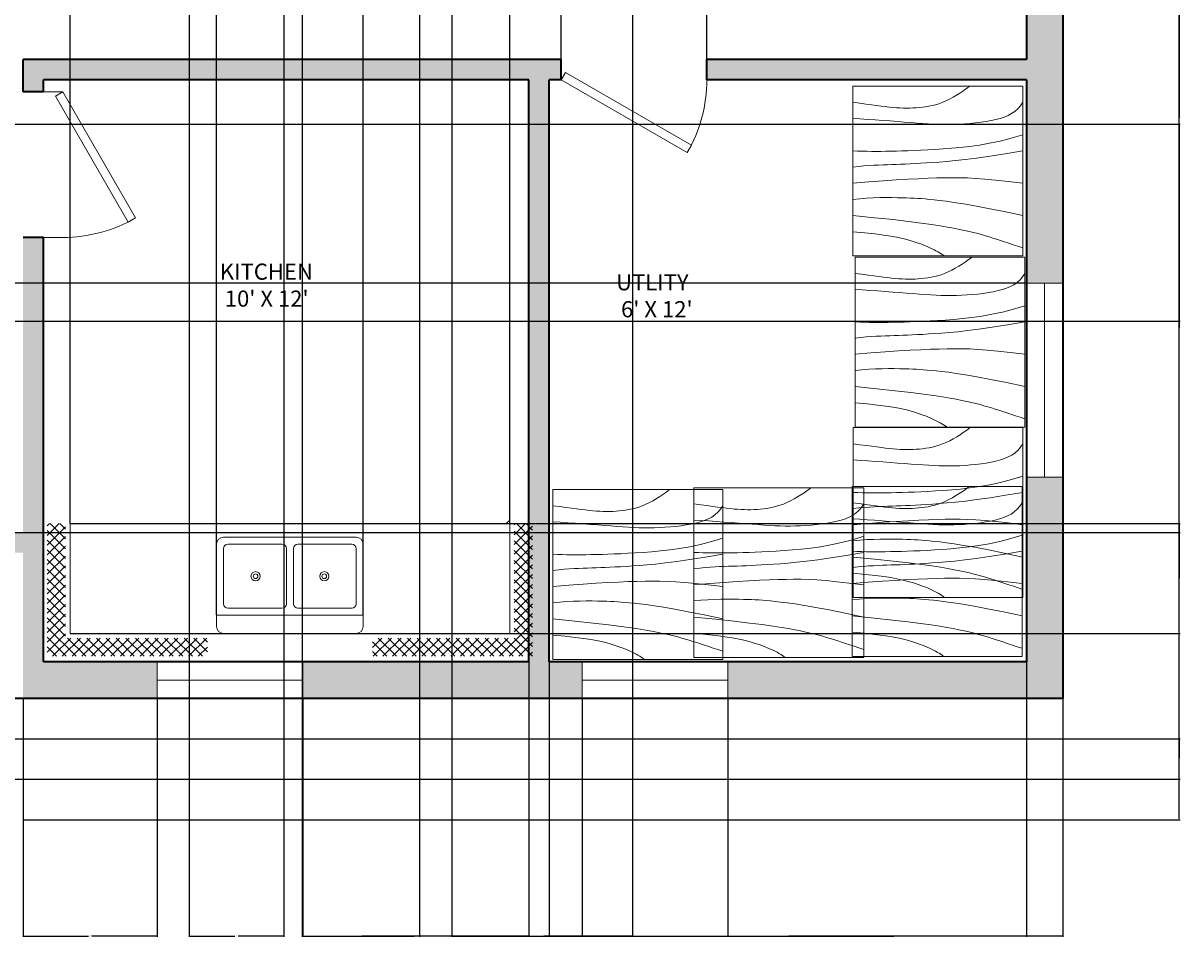
# Model space of a CAD drawing. Units: inches. Extents: x -28 to 649, y -11 to 509.
# Tile 5 of 7: x 346 to 633, y -11 to 215. Entities that reach past the tile are written whole.
import ezdxf

# ---------------------------------------------------------------- set-up
doc = ezdxf.new("R2010")
doc.units = ezdxf.units.IN
doc.header["$MEASUREMENT"] = 0
for name, color, linetype, lineweight in [('A-ANNO-DIMS', 2, 'Continuous', 18), ('A-AREA-IDEN', 18, 'Continuous', 18), ('A-FLOR-CASE', 4, 'Continuous', 20), ('A-FLOR-CASE-PATT', 181, 'Continuous', 13), ('A-FLOR-FIXT', 181, 'Continuous', 18), ('A-WALL', 7, 'Continuous', 35), ('A-WALL-PATT', 251, 'Continuous', 13), ('doors', 40, 'Continuous', 20), ('window', 30, 'Continuous', 18)]:
    doc.layers.add(name, color=color, linetype=linetype, lineweight=lineweight)
doc.styles.get("Standard").update_dxf_attribs({"font": 'arial.ttf'})
doc.dimstyles.get("Standard").update_dxf_attribs({"dimtxt": 0.18, "dimasz": 0.18, "dimexe": 0.18, "dimexo": 0.0625, "dimgap": 0.09, "dimtad": 0, "dimtih": 1, "dimtoh": 1, "dimdec": 4, "dimzin": 0, "dimdsep": 46, "dimtxsty": 'Standard', "dimcen": 0.09, "dimadec": 0, "dimazin": 0, "dimtfac": 1, "dimtdec": 4, "dimtofl": 0, "dimtmove": 0, "dimatfit": 3, "dimfxl": 1, "dimtolj": 1, "dimtzin": 0, "dimarcsym": 0})

# ---------------------------------------------------------------- blocks, each defined once
blk = doc.blocks.new('*U9')
for p, q in [((0, 0), (0, -100)), ((750, 0), (750, -100))]:
    blk.add_line(p, q)
blk.add_lwpolyline([(0, 0), (649.5, 375), (671.4, 337.1), (21.9, -37.9)], close=True)
blk.add_arc((0, 0), 750, 0, 30)
blk = doc.blocks.new('*U10')
for p, q in [((0, 0), (0, 100)), ((750, 0), (750, 100))]:
    blk.add_line(p, q)
blk.add_lwpolyline([(0, 0), (649.5, -375), (671.4, -337.1), (21.9, 37.9)], close=True)
blk.add_arc((0, 0), 750, 330, 0)
blk = doc.blocks.new('Table - Square Woodgrain 42 x 42 in.')
blk.add_line((0, -42), (42, -42))
for points in [[(0, -4), (1.704, -4.2172), (3.2358, -4.4188), (4.615, -4.604), (5.8615, -4.7721), (6.9951, -4.9224), (8.0357, -5.0541), (9.0031, -5.1667), (9.9171, -5.2594), (10.7951, -5.3316), (11.6445, -5.3836), (12.4702, -5.4157), (13.277, -5.4283), (14.0698, -5.4217), (14.8535, -5.3964), (15.6331, -5.3526), (16.4133, -5.2908), (17.1986, -5.2103), (17.9913, -5.1062), (18.793, -4.9727), (19.6056, -4.8038), (20.4307, -4.5937), (21.2701, -4.3365), (22.1256, -4.0262), (22.9989, -3.6571), (23.888, -3.2272), (24.7756, -2.7516), (25.6408, -2.2491), (26.4624, -1.7387), (27.2195, -1.2395), (27.891, -0.7703), (28.456, -0.3501), (28.8934, 0.002)], [(0, -42), (0, 0), (42, 0), (42, -42)], [(0, -8), (1.8203, -8.1001), (3.6741, -8.2149), (5.5411, -8.3408), (7.4011, -8.4741), (9.2339, -8.6112), (11.0193, -8.7484), (12.7371, -8.8821), (14.3671, -9.0086), (15.8954, -9.1246), (17.3337, -9.2278), (18.6997, -9.3159), (20.0116, -9.387), (21.2871, -9.4389), (22.5442, -9.4696), (23.8008, -9.477), (25.0749, -9.459), (26.3791, -9.4137), (27.7049, -9.3403), (29.0383, -9.2382), (30.3655, -9.1068), (31.6728, -8.9455), (32.9461, -8.7535), (34.1717, -8.5304), (35.3358, -8.2756), (36.4268, -7.9863), (37.443, -7.6521), (38.3849, -7.2603), (39.253, -6.7986), (40.048, -6.2542), (40.7705, -5.6147), (41.421, -4.8674), (42, -4)], [(42, -12), (39.1784, -12.8621), (36.4519, -13.5654), (33.8246, -14.1294), (31.3004, -14.5731), (28.8832, -14.9161), (26.577, -15.1775), (24.3858, -15.3768), (22.3136, -15.5332), (20.3622, -15.6632), (18.5254, -15.7718), (16.7947, -15.8612), (15.1618, -15.9338), (13.6183, -15.9916), (12.1558, -16.0369), (10.7659, -16.0718), (9.4403, -16.0987), (8.1703, -16.1191), (6.9461, -16.1325), (5.7577, -16.1377), (4.595, -16.1335), (3.4479, -16.1188), (2.3064, -16.0924), (1.1604, -16.0532), (0, -16)], [(42, -16), (37.6529, -16.7365), (33.8802, -17.329), (30.6179, -17.7961), (27.8015, -18.1561), (25.3668, -18.4275), (23.2497, -18.6288), (21.3859, -18.7785), (19.7111, -18.8949), (18.1693, -18.9939), (16.7375, -19.0795), (15.401, -19.1534), (14.1449, -19.217), (12.9544, -19.2717), (11.8148, -19.3191), (10.7113, -19.3606), (9.6291, -19.3976), (8.5534, -19.4323), (7.47, -19.4689), (6.3643, -19.5122), (5.222, -19.5672), (4.0288, -19.6386), (2.7703, -19.7313), (1.4321, -19.8501), (0, -20)], [(0, -24), (3.9243, -23.6805), (7.4766, -23.4138), (10.6891, -23.1954), (13.5943, -23.0205), (16.2247, -22.8847), (18.6125, -22.7832), (20.7903, -22.7116), (22.7903, -22.6651), (24.6563, -22.642), (26.4764, -22.6507), (28.35, -22.7024), (30.3766, -22.8084), (32.6555, -22.98), (35.2861, -23.2283), (38.3678, -23.5645), (42, -24)], [(42, -32), (37.392, -31.017), (33.4585, -30.2231), (30.1291, -29.5949), (27.3334, -29.109), (25.0009, -28.742), (23.0612, -28.4707), (21.4439, -28.2716), (20.0786, -28.1215), (18.8998, -28.0002), (17.8609, -27.9014), (16.9206, -27.8219), (16.0371, -27.7588), (15.1691, -27.709), (14.2748, -27.6693), (13.3128, -27.6368), (12.2415, -27.6083), (11.0295, -27.5824), (9.6867, -27.5643), (8.233, -27.5608), (6.6884, -27.5787), (5.0728, -27.6248), (3.4062, -27.7058), (1.7086, -27.8286), (0, -28)], [(0, -32), (5.4026, -32.5358), (9.9494, -33.019), (13.7424, -33.4553), (16.8834, -33.8505), (19.4743, -34.2106), (21.6171, -34.5413), (23.4136, -34.8486), (24.9657, -35.1382), (26.3614, -35.4156), (27.6332, -35.6841), (28.7995, -35.9467), (29.8788, -36.2064), (30.8897, -36.4661), (31.8507, -36.7288), (32.7802, -36.9973), (33.6968, -37.2747), (34.6175, -37.5635), (35.5531, -37.8651), (36.5128, -38.1805), (37.506, -38.5108), (38.5421, -38.8568), (39.6302, -39.2197), (40.7797, -39.6004), (42, -40)], [(0, -36), (3.0098, -36.2857), (5.5354, -36.5643), (7.6368, -36.8359), (9.374, -37.1009), (10.807, -37.3597), (11.9957, -37.6126), (13.0002, -37.8599), (13.8804, -38.102), (14.6874, -38.3393), (15.4365, -38.5729), (16.1338, -38.8041), (16.7858, -39.0341), (17.3987, -39.264), (17.9787, -39.4952), (18.5322, -39.7288), (19.0655, -39.9662), (19.5832, -40.2081), (20.0842, -40.4544), (20.5657, -40.7046), (21.0249, -40.9581), (21.459, -41.2144), (21.8653, -41.4731), (22.2409, -41.7335), (22.5831, -41.9951)]]:
    blk.add_lwpolyline(points)
blk = doc.blocks.new('WIN-48x9')
for p, q in [((9, 48), (0, 48)), ((0, 48), (0, 0)), ((4.5, 0), (4.5, 48)), ((9, 0), (9, 48)), ((0, 0), (9, 0)), ((0, 0), (4.5, 0))]:
    blk.add_line(p, q)
blk = doc.blocks.new('WIN-36x9')
for p, q in [((0, 9), (0, 0)), ((36, 9), (0, 9)), ((0, 9), (0, 4.5)), ((36, 0), (36, 9)), ((0, 4.5), (36, 4.5)), ((0, 0), (36, 0))]:
    blk.add_line(p, q)
blk = doc.blocks.new('*D31')
at = {"layer": 'A-ANNO-DIMS', "color": 0, "lineweight": -2, "transparency": 16777216}
for p, q in [((603.51, 479.94), (632.43, 479.94)), ((632.25, 479.76), (632.25, 249.12)), ((632.25, 18.12), (632.25, 248.76)), ((346.51, 17.94), (632.43, 17.94))]:
    blk.add_line(p, q, dxfattribs=at)
at = {"layer": 'A-ANNO-DIMS', "color": 0, "transparency": 16777216}
for points in [[(632.22, 479.76), (632.28, 479.76), (632.25, 479.94)], [(632.22, 18.12), (632.28, 18.12), (632.25, 17.94)]]:
    blk.add_solid(points, dxfattribs=at)
at = {"layer": 'Defpoints', "color": 0, "transparency": 16777216}
for p in [(603.45, 479.94), (632.25, 479.94), (346.45, 17.94)]:
    blk.add_point(p, dxfattribs=at)
at = {"layer": 'A-ANNO-DIMS', "color": 0, "transparency": 16777216, "insert": (632.25, 248.94), "char_height": 0.18, "attachment_point": 5}
blk.add_mtext('\\A1;462', dxfattribs=at)
blk = doc.blocks.new('*D33')
at = {"layer": 'A-ANNO-DIMS', "color": 0, "lineweight": -2, "transparency": 16777216}
for p, q in [((280.51, 37.94), (632.43, 37.94)), ((632.25, 37.76), (632.25, 33.12)), ((632.25, 28.12), (632.25, 32.76)), ((280.51, 27.94), (632.43, 27.94))]:
    blk.add_line(p, q, dxfattribs=at)
at = {"layer": 'A-ANNO-DIMS', "color": 0, "transparency": 16777216}
for points in [[(632.22, 37.76), (632.28, 37.76), (632.25, 37.94)], [(632.22, 28.12), (632.28, 28.12), (632.25, 27.94)]]:
    blk.add_solid(points, dxfattribs=at)
at = {"layer": 'Defpoints', "color": 0, "transparency": 16777216}
for p in [(280.45, 37.94), (632.25, 37.94), (280.45, 27.94)]:
    blk.add_point(p, dxfattribs=at)
at = {"layer": 'A-ANNO-DIMS', "color": 0, "transparency": 16777216, "insert": (632.25, 32.94), "char_height": 0.18, "attachment_point": 5}
blk.add_mtext('\\A1;10', dxfattribs=at)
blk = doc.blocks.new('*D40')
at = {"layer": 'A-ANNO-DIMS', "color": 0, "lineweight": -2, "transparency": 16777216}
for p, q in [((346.45, 47.88), (346.45, -11.04)), ((379.58, 47.88), (379.58, -11.04)), ((346.63, -10.86), (362.62, -10.86)), ((379.4, -10.86), (363.41, -10.86))]:
    blk.add_line(p, q, dxfattribs=at)
at = {"layer": 'A-ANNO-DIMS', "color": 0, "transparency": 16777216}
for points in [[(346.63, -10.83), (346.63, -10.89), (346.45, -10.86)], [(379.4, -10.83), (379.4, -10.89), (379.58, -10.86)]]:
    blk.add_solid(points, dxfattribs=at)
at = {"layer": 'Defpoints', "color": 0, "transparency": 16777216}
for p in [(346.45, 47.94), (379.58, 47.94), (379.58, -10.86)]:
    blk.add_point(p, dxfattribs=at)
at = {"layer": 'A-ANNO-DIMS', "color": 0, "transparency": 16777216, "insert": (363.01, -10.86), "char_height": 0.18, "attachment_point": 5}
blk.add_mtext('\\A1;33.13', dxfattribs=at)
blk = doc.blocks.new('*D41')
at = {"layer": 'A-ANNO-DIMS', "color": 0, "lineweight": -2, "transparency": 16777216}
for p, q in [((471.45, 56.88), (471.45, -11.04)), ((415.58, 47.88), (415.58, -11.04)), ((415.76, -10.86), (443.12, -10.86)), ((471.27, -10.86), (443.91, -10.86))]:
    blk.add_line(p, q, dxfattribs=at)
at = {"layer": 'A-ANNO-DIMS', "color": 0, "transparency": 16777216}
for points in [[(415.76, -10.83), (415.76, -10.89), (415.58, -10.86)], [(471.27, -10.83), (471.27, -10.89), (471.45, -10.86)]]:
    blk.add_solid(points, dxfattribs=at)
at = {"layer": 'Defpoints', "color": 0, "transparency": 16777216}
for p in [(471.45, 56.94), (415.58, 47.94), (471.45, -10.86)]:
    blk.add_point(p, dxfattribs=at)
at = {"layer": 'A-ANNO-DIMS', "color": 0, "transparency": 16777216, "insert": (443.51, -10.86), "char_height": 0.18, "attachment_point": 5}
blk.add_mtext('\\A1;55.87', dxfattribs=at)
blk = doc.blocks.new('*D42')
at = {"layer": 'A-ANNO-DIMS', "color": 0, "lineweight": -2, "transparency": 16777216}
for p, q in [((471.45, 56.88), (471.45, -11.04)), ((484.62, 47.88), (484.62, -11.04)), ((471.63, -10.86), (477.58, -10.86)), ((484.44, -10.86), (478.49, -10.86))]:
    blk.add_line(p, q, dxfattribs=at)
at = {"layer": 'A-ANNO-DIMS', "color": 0, "transparency": 16777216}
for points in [[(471.63, -10.83), (471.63, -10.89), (471.45, -10.86)], [(484.44, -10.83), (484.44, -10.89), (484.62, -10.86)]]:
    blk.add_solid(points, dxfattribs=at)
at = {"layer": 'Defpoints', "color": 0, "transparency": 16777216}
for p in [(471.45, 56.94), (484.62, 47.94), (484.62, -10.86)]:
    blk.add_point(p, dxfattribs=at)
at = {"layer": 'A-ANNO-DIMS', "color": 0, "transparency": 16777216, "insert": (478.03, -10.86), "char_height": 0.18, "attachment_point": 5}
blk.add_mtext('\\A1;13.168', dxfattribs=at)
blk = doc.blocks.new('*D43')
at = {"layer": 'A-ANNO-DIMS', "color": 0, "lineweight": -2, "transparency": 16777216}
for p, q in [((520.62, 47.88), (520.62, -11.04)), ((603.45, 47.88), (603.45, -11.04)), ((520.8, -10.86), (561.64, -10.86)), ((603.27, -10.86), (562.43, -10.86))]:
    blk.add_line(p, q, dxfattribs=at)
at = {"layer": 'A-ANNO-DIMS', "color": 0, "transparency": 16777216}
for points in [[(520.8, -10.83), (520.8, -10.89), (520.62, -10.86)], [(603.27, -10.83), (603.27, -10.89), (603.45, -10.86)]]:
    blk.add_solid(points, dxfattribs=at)
at = {"layer": 'Defpoints', "color": 0, "transparency": 16777216}
for p in [(520.62, 47.94), (603.45, 47.94), (603.45, -10.86)]:
    blk.add_point(p, dxfattribs=at)
at = {"layer": 'A-ANNO-DIMS', "color": 0, "transparency": 16777216, "insert": (562.03, -10.86), "char_height": 0.18, "attachment_point": 5}
blk.add_mtext('\\A1;82.83', dxfattribs=at)
blk = doc.blocks.new('*D47')
at = {"layer": 'A-ANNO-DIMS', "color": 0, "lineweight": -2, "transparency": 16777216}
for p, q in [((387.45, 470.88), (387.45, -11.04)), ((410.91, 470.88), (410.91, -11.04)), ((387.63, -10.86), (398.79, -10.86)), ((410.73, -10.86), (399.58, -10.86))]:
    blk.add_line(p, q, dxfattribs=at)
at = {"layer": 'A-ANNO-DIMS', "color": 0, "transparency": 16777216}
for points in [[(387.63, -10.83), (387.63, -10.89), (387.45, -10.86)], [(410.73, -10.83), (410.73, -10.89), (410.91, -10.86)]]:
    blk.add_solid(points, dxfattribs=at)
at = {"layer": 'Defpoints', "color": 0, "transparency": 16777216}
for p in [(387.45, 470.94), (410.91, 470.94), (410.91, -10.86)]:
    blk.add_point(p, dxfattribs=at)
at = {"layer": 'A-ANNO-DIMS', "color": 0, "transparency": 16777216, "insert": (399.18, -10.86), "char_height": 0.18, "attachment_point": 5}
blk.add_mtext('\\A1;23.46', dxfattribs=at)
blk = doc.blocks.new('*D48')
at = {"layer": 'A-ANNO-DIMS', "color": 0, "lineweight": -2, "transparency": 16777216}
for p, q in [((452.45, 470.88), (452.45, -11.04)), ((497.1, 470.88), (497.1, -11.04)), ((452.63, -10.86), (474.38, -10.86)), ((496.92, -10.86), (475.17, -10.86))]:
    blk.add_line(p, q, dxfattribs=at)
at = {"layer": 'A-ANNO-DIMS', "color": 0, "transparency": 16777216}
for points in [[(452.63, -10.83), (452.63, -10.89), (452.45, -10.86)], [(496.92, -10.83), (496.92, -10.89), (497.1, -10.86)]]:
    blk.add_solid(points, dxfattribs=at)
at = {"layer": 'Defpoints', "color": 0, "transparency": 16777216}
for p in [(452.45, 470.94), (497.1, 470.94), (497.1, -10.86)]:
    blk.add_point(p, dxfattribs=at)
at = {"layer": 'A-ANNO-DIMS', "color": 0, "transparency": 16777216, "insert": (474.77, -10.86), "char_height": 0.18, "attachment_point": 5}
blk.add_mtext('\\A1;44.65', dxfattribs=at)
blk = doc.blocks.new('*D52')
at = {"layer": 'A-ANNO-DIMS', "color": 0, "lineweight": -2, "transparency": 16777216}
for p, q in [((594.39, 262.25), (-1.53, 262.25)), ((-1.35, 262.07), (-1.35, 206.61)), ((-1.35, 150.79), (-1.35, 206.25)), ((594.39, 150.61), (-1.53, 150.61))]:
    blk.add_line(p, q, dxfattribs=at)
at = {"layer": 'A-ANNO-DIMS', "color": 0, "transparency": 16777216}
for points in [[(-1.38, 262.07), (-1.32, 262.07), (-1.35, 262.25)], [(-1.38, 150.79), (-1.32, 150.79), (-1.35, 150.61)]]:
    blk.add_solid(points, dxfattribs=at)
at = {"layer": 'Defpoints', "color": 0, "transparency": 16777216}
for p in [(-1.35, 262.25), (594.45, 262.25), (594.45, 150.61)]:
    blk.add_point(p, dxfattribs=at)
at = {"layer": 'A-ANNO-DIMS', "color": 0, "transparency": 16777216, "insert": (-1.35, 206.43), "char_height": 0.18, "attachment_point": 5}
blk.add_mtext('\\A1;111.64', dxfattribs=at)
blk = doc.blocks.new('*D53')
at = {"layer": 'A-ANNO-DIMS', "color": 0, "lineweight": -2, "transparency": 16777216}
for p, q in [((36.51, 241.9), (632.43, 241.9)), ((632.25, 241.72), (632.25, 191.76)), ((632.25, 141.44), (632.25, 191.39)), ((36.51, 141.26), (632.43, 141.26))]:
    blk.add_line(p, q, dxfattribs=at)
at = {"layer": 'A-ANNO-DIMS', "color": 0, "transparency": 16777216}
for points in [[(632.22, 241.72), (632.28, 241.72), (632.25, 241.9)], [(632.22, 141.44), (632.28, 141.44), (632.25, 141.26)]]:
    blk.add_solid(points, dxfattribs=at)
at = {"layer": 'Defpoints', "color": 0, "transparency": 16777216}
for p in [(36.45, 241.9), (632.25, 241.9), (36.45, 141.26)]:
    blk.add_point(p, dxfattribs=at)
at = {"layer": 'A-ANNO-DIMS', "color": 0, "transparency": 16777216, "insert": (632.25, 191.58), "char_height": 0.18, "attachment_point": 5}
blk.add_mtext('\\A1;100.64', dxfattribs=at)
blk = doc.blocks.new('*D60')
at = {"layer": 'A-ANNO-DIMS', "color": 0, "lineweight": -2, "transparency": 16777216}
for p, q in [((479.45, 206), (479.45, 508.92)), ((479.63, 508.74), (497.23, 508.74)), ((515.27, 508.74), (497.67, 508.74)), ((515.45, 206), (515.45, 508.92))]:
    blk.add_line(p, q, dxfattribs=at)
at = {"layer": 'A-ANNO-DIMS', "color": 0, "transparency": 16777216}
for points in [[(479.63, 508.77), (479.63, 508.71), (479.45, 508.74)], [(515.27, 508.77), (515.27, 508.71), (515.45, 508.74)]]:
    blk.add_solid(points, dxfattribs=at)
at = {"layer": 'Defpoints', "color": 0, "transparency": 16777216}
for p in [(515.45, 508.74), (479.45, 205.94), (515.45, 205.94)]:
    blk.add_point(p, dxfattribs=at)
at = {"layer": 'A-ANNO-DIMS', "color": 0, "transparency": 16777216, "insert": (497.45, 508.74), "char_height": 0.18, "attachment_point": 5}
blk.add_mtext('\\A1;36', dxfattribs=at)
blk = doc.blocks.new('*D61')
at = {"layer": 'A-ANNO-DIMS', "color": 0, "lineweight": -2, "transparency": 16777216}
for p, q in [((274.51, 189.94), (632.43, 189.94)), ((632.25, 189.76), (632.25, 139.62)), ((632.25, 89.12), (632.25, 139.26)), ((274.51, 88.94), (632.43, 88.94))]:
    blk.add_line(p, q, dxfattribs=at)
at = {"layer": 'A-ANNO-DIMS', "color": 0, "transparency": 16777216}
for points in [[(632.22, 189.76), (632.28, 189.76), (632.25, 189.94)], [(632.22, 89.12), (632.28, 89.12), (632.25, 88.94)]]:
    blk.add_solid(points, dxfattribs=at)
at = {"layer": 'Defpoints', "color": 0, "transparency": 16777216}
for p in [(274.45, 189.94), (632.25, 189.94), (274.45, 88.94)]:
    blk.add_point(p, dxfattribs=at)
at = {"layer": 'A-ANNO-DIMS', "color": 0, "transparency": 16777216, "insert": (632.25, 139.44), "char_height": 0.18, "attachment_point": 5}
blk.add_mtext('\\A1;101', dxfattribs=at)
blk = doc.blocks.new('*D63')
at = {"layer": 'A-ANNO-DIMS', "color": 0, "lineweight": -2, "transparency": 16777216}
for p, q in [((415.45, 381.88), (415.45, -11.04)), ((444.45, 381.88), (444.45, -11.04)), ((415.63, -10.86), (429.73, -10.86)), ((444.27, -10.86), (430.17, -10.86))]:
    blk.add_line(p, q, dxfattribs=at)
at = {"layer": 'A-ANNO-DIMS', "color": 0, "transparency": 16777216}
for points in [[(415.63, -10.83), (415.63, -10.89), (415.45, -10.86)], [(444.27, -10.83), (444.27, -10.89), (444.45, -10.86)]]:
    blk.add_solid(points, dxfattribs=at)
at = {"layer": 'Defpoints', "color": 0, "transparency": 16777216}
for p in [(415.45, 381.94), (444.45, 381.94), (444.45, -10.86)]:
    blk.add_point(p, dxfattribs=at)
at = {"layer": 'A-ANNO-DIMS', "color": 0, "transparency": 16777216, "insert": (429.95, -10.86), "char_height": 0.18, "attachment_point": 5}
blk.add_mtext('\\A1;29', dxfattribs=at)
blk = doc.blocks.new('*D68')
at = {"layer": 'A-ANNO-DIMS', "color": 0, "lineweight": -2, "transparency": 16777216}
for p, q in [((358.05, 91.23), (358.05, 508.92)), ((358.23, 508.74), (411.94, 508.74)), ((466.55, 508.74), (412.85, 508.74)), ((466.73, 91.23), (466.73, 508.92))]:
    blk.add_line(p, q, dxfattribs=at)
at = {"layer": 'A-ANNO-DIMS', "color": 0, "transparency": 16777216}
for points in [[(358.23, 508.77), (358.23, 508.71), (358.05, 508.74)], [(466.55, 508.77), (466.55, 508.71), (466.73, 508.74)]]:
    blk.add_solid(points, dxfattribs=at)
at = {"layer": 'Defpoints', "color": 0, "transparency": 16777216}
for p in [(466.73, 508.74), (358.05, 91.17), (466.73, 91.17)]:
    blk.add_point(p, dxfattribs=at)
at = {"layer": 'A-ANNO-DIMS', "color": 0, "transparency": 16777216, "insert": (412.39, 508.74), "char_height": 0.18, "attachment_point": 5}
blk.add_mtext('\\A1;108.68', dxfattribs=at)
blk = doc.blocks.new('*D69')
at = {"layer": 'A-ANNO-DIMS', "color": 0, "lineweight": -2, "transparency": 16777216}
for p, q in [((358.11, 91.17), (632.43, 91.17)), ((632.25, 90.99), (632.25, 77.76)), ((632.25, 64.18), (632.25, 77.4)), ((358.11, 64), (632.43, 64))]:
    blk.add_line(p, q, dxfattribs=at)
at = {"layer": 'A-ANNO-DIMS', "color": 0, "transparency": 16777216}
for points in [[(632.22, 90.99), (632.28, 90.99), (632.25, 91.17)], [(632.22, 64.18), (632.28, 64.18), (632.25, 64)]]:
    blk.add_solid(points, dxfattribs=at)
at = {"layer": 'Defpoints', "color": 0, "transparency": 16777216}
for p in [(358.05, 91.17), (632.25, 91.17), (358.05, 64)]:
    blk.add_point(p, dxfattribs=at)
at = {"layer": 'A-ANNO-DIMS', "color": 0, "transparency": 16777216, "insert": (632.25, 77.58), "char_height": 0.18, "attachment_point": 5}
blk.add_mtext('\\A1;27.17', dxfattribs=at)
blk = doc.blocks.new('*D70')
at = {"layer": 'A-ANNO-DIMS', "color": 0, "lineweight": -2, "transparency": 16777216}
for p, q in [((394.28, 68.59), (394.28, 508.92)), ((394.46, 508.74), (412, 508.74)), ((430.33, 508.74), (412.79, 508.74)), ((430.51, 68.59), (430.51, 508.92))]:
    blk.add_line(p, q, dxfattribs=at)
at = {"layer": 'A-ANNO-DIMS', "color": 0, "transparency": 16777216}
for points in [[(394.46, 508.77), (394.46, 508.71), (394.28, 508.74)], [(430.33, 508.77), (430.33, 508.71), (430.51, 508.74)]]:
    blk.add_solid(points, dxfattribs=at)
at = {"layer": 'Defpoints', "color": 0, "transparency": 16777216}
for p in [(430.51, 508.74), (394.28, 68.53), (430.51, 68.53)]:
    blk.add_point(p, dxfattribs=at)
at = {"layer": 'A-ANNO-DIMS', "color": 0, "transparency": 16777216, "insert": (412.39, 508.74), "char_height": 0.18, "attachment_point": 5}
blk.add_mtext('\\A1;36.23', dxfattribs=at)
blk = doc.blocks.new('*D71')
at = {"layer": 'A-ANNO-DIMS', "color": 0, "lineweight": -2, "transparency": 16777216}
for p, q in [((476.45, 56.88), (476.45, -11.04)), ((594.45, 56.88), (594.45, -11.04)), ((476.63, -10.86), (535.17, -10.86)), ((594.27, -10.86), (535.73, -10.86))]:
    blk.add_line(p, q, dxfattribs=at)
at = {"layer": 'A-ANNO-DIMS', "color": 0, "transparency": 16777216}
for points in [[(476.63, -10.83), (476.63, -10.89), (476.45, -10.86)], [(594.27, -10.83), (594.27, -10.89), (594.45, -10.86)]]:
    blk.add_solid(points, dxfattribs=at)
at = {"layer": 'Defpoints', "color": 0, "transparency": 16777216}
for p in [(476.45, 56.94), (594.45, 56.94), (594.45, -10.86)]:
    blk.add_point(p, dxfattribs=at)
at = {"layer": 'A-ANNO-DIMS', "color": 0, "transparency": 16777216, "insert": (535.45, -10.86), "char_height": 0.18, "attachment_point": 5}
blk.add_mtext('\\A1;118', dxfattribs=at)

msp = doc.modelspace()

# ---------------------------------------------------------------- hatches: boundary and pattern name
at = {"layer": 'A-FLOR-CASE-PATT'}
h = msp.add_hatch(dxfattribs=at)
h.set_pattern_fill('ANSI37', color=256, scale=13.5849, style=0)
h.paths.add_polyline_path([(352.3918, 58.3392), (392.0145, 58.3392), (392.0145, 62.8675), (356.9201, 62.8675), (356.9201, 91.1694), (352.3918, 91.1694)])
h = msp.add_hatch(dxfattribs=at)
h.set_pattern_fill('ANSI37', color=256, scale=13.5849, style=0)
h.paths.add_polyline_path([(432.7692, 58.3392), (472.3918, 58.3392), (472.3918, 91.1694), (467.8635, 91.1694), (467.8635, 62.8675), (432.7692, 62.8675)])
at = {"layer": 'A-WALL-PATT'}
h = msp.add_hatch(color=256, dxfattribs=at)
h.dxf.hatch_style = 1
h.paths.add_polyline_path([(36.4499, 184.9382), (165.4499, 184.9382), (165.4499, 189.9382), (36.4499, 189.9382), (36.4499, 241.898), (27.4499, 241.898), (27.4499, 141.2558), (36.4499, 141.2558)])
h.paths.add_polyline_path([(36.4499, 385.8835), (27.4499, 385.8835), (27.4499, 289.898), (36.4499, 289.898)])
h.paths.add_polyline_path([(185.4499, 341.9382), (180.4499, 341.9382), (180.4499, 338.9382), (36.4499, 338.9382), (36.4499, 333.9382), (185.4499, 333.9382)])
h.paths.add_polyline_path([(36.4499, 470.9382), (79.2168, 470.9382), (79.2168, 479.9382), (27.4499, 479.9382), (27.4499, 433.8835), (36.4499, 433.8835)])
h.paths.add_polyline_path([(185.4499, 470.9382), (203.9104, 470.9382), (203.9104, 479.9382), (127.2168, 479.9382), (127.2168, 470.9382), (180.4499, 470.9382), (180.4499, 381.9382), (188.4499, 381.9382), (188.4499, 386.9382), (185.4499, 386.9382)])
h.paths.add_polyline_path([(292.4601, 479.9382), (227.9104, 479.9382), (227.9104, 470.9382), (245.4499, 470.9382), (245.4499, 386.9382), (217.4499, 386.9382), (217.4499, 381.9382), (245.4499, 381.9382), (245.4499, 338.9382), (245.4499, 333.9382), (251.5222, 333.9382), (251.5222, 338.9382), (250.4499, 338.9382), (250.4499, 470.9382), (292.4601, 470.9382)])
h.paths.add_polyline_path([(410.9121, 479.9382), (340.4601, 479.9382), (340.4601, 470.9382), (382.4499, 470.9382), (382.4499, 338.9382), (287.5222, 338.9382), (287.5222, 333.9382), (387.4499, 333.9382), (387.4499, 381.9382), (415.4499, 381.9382), (415.4499, 386.9382), (387.4499, 386.9382), (387.4499, 470.9382), (410.9121, 470.9382)])
h.paths.add_polyline_path([(497.0961, 479.9382), (434.9121, 479.9382), (434.9121, 470.9382), (447.4499, 470.9382), (447.4499, 386.9382), (444.4499, 386.9382), (444.4499, 381.9382), (452.4499, 381.9382), (452.4499, 470.9382), (497.0961, 470.9382)])
h.paths.add_polyline_path([(603.4499, 479.9382), (545.0961, 479.9382), (545.0961, 470.9382), (594.4499, 470.9382), (594.4499, 418.4819), (603.4499, 418.4819)])
h.paths.add_polyline_path([(603.4499, 370.4819), (594.4499, 370.4819), (594.4499, 338.9382), (452.4499, 338.9382), (452.4499, 341.9382), (447.4499, 341.9382), (447.4499, 338.9382), (447.4499, 333.9382), (594.4499, 333.9382), (594.4499, 310.2528), (603.4499, 310.2528)])
h.paths.add_polyline_path([(603.4499, 262.2528), (594.4499, 262.2528), (594.4499, 205.9382), (515.4499, 205.9382), (515.4499, 200.9382), (594.4499, 200.9382), (594.4499, 150.6102), (603.4499, 150.6102)])
h = msp.add_hatch(color=256, dxfattribs=at)
h.dxf.hatch_style = 1
h.paths.add_polyline_path([(603.4499, 102.6102), (594.4499, 102.6102), (594.4499, 56.9382), (520.6175, 56.9382), (520.6175, 47.9382), (603.4499, 47.9382)])
h.paths.add_polyline_path([(484.6175, 56.9382), (476.4499, 56.9382), (476.4499, 200.9382), (479.4499, 200.9382), (479.4499, 205.9382), (346.4499, 205.9382), (346.4499, 197.9382), (351.4499, 197.9382), (351.4499, 200.9382), (471.4499, 200.9382), (471.4499, 56.9382), (415.5771, 56.9382), (415.5771, 47.9382), (484.6175, 47.9382)])
h.paths.add_polyline_path([(379.5771, 56.9382), (351.4499, 56.9382), (351.4499, 161.9382), (346.4499, 161.9382), (346.4499, 88.9382), (334.4499, 88.9382), (334.4499, 83.9382), (346.4499, 83.9382), (346.4499, 47.9382), (379.5771, 47.9382)])

# ---------------------------------------------------------------- linework, layer by layer
at = {"layer": 'A-FLOR-CASE'}
msp.add_lwpolyline([(466.7314, 91.1694), (466.7314, 63.9996), (358.0522, 63.9996), (358.0522, 91.1694)], close=True, dxfattribs=at)
at = {"layer": 'A-FLOR-CASE-PATT'}
msp.add_line((465.8821, 91.1694), (466.7314, 92.0187), dxfattribs=at)
at = {"layer": 'A-FLOR-FIXT'}
msp.add_line((430.505, 68.5279), (394.2786, 68.5279), dxfattribs=at)
for points in [[(430.505, 65.6977, -0.41421356), (428.8069, 63.9996), (395.9767, 63.9996, -0.41421356), (394.2786, 65.6977), (394.2786, 86.075, -0.41421356), (395.9767, 87.7732), (428.8069, 87.7732, -0.41421356), (430.505, 86.075)], [(397.1088, 70.226, -0.41421356), (395.9767, 71.3581), (395.9767, 84.943, -0.41421356), (397.1088, 86.075), (410.4107, 86.075, -0.41421356), (411.5428, 84.943), (411.5428, 71.3581, -0.41421356), (410.4107, 70.226)], [(413.2409, 84.943, -0.41421356), (414.3729, 86.075), (427.6748, 86.075, -0.41421356), (428.8069, 84.943), (428.8069, 71.3581, -0.41421356), (427.6748, 70.226), (414.3729, 70.226, -0.41421356), (413.2409, 71.3581)]]:
    msp.add_lwpolyline(points, format="xyb", close=True, dxfattribs=at)
for centre, radius in [((403.9012, 78.1505), 1.1321), ((403.9012, 78.1505), 0.566), ((420.8824, 78.1505), 1.1321), ((420.8824, 78.1505), 0.566)]:
    msp.add_circle(centre, radius, dxfattribs=at)
at = {"layer": 'A-WALL'}
for p, q in [((594.4499, 333.9382), (594.4499, 205.9382)), ((479.4499, 205.9382), (346.4499, 205.9382)), ((346.4499, 197.9382), (346.4499, 205.9382)), ((479.4499, 200.9382), (479.4499, 205.9382)), ((594.4499, 205.9382), (515.4499, 205.9382)), ((515.4499, 200.9382), (515.4499, 205.9382)), ((471.4499, 200.9382), (351.4499, 200.9382)), ((351.4499, 197.9382), (351.4499, 200.9382)), ((471.4499, 56.9382), (471.4499, 200.9382)), ((479.4499, 200.9382), (476.4499, 200.9382)), ((476.4499, 56.9382), (476.4499, 200.9382)), ((594.4499, 200.9382), (515.4499, 200.9382)), ((594.4499, 200.9382), (594.4499, 56.9382)), ((351.4499, 197.9382), (346.4499, 197.9382)), ((351.4499, 161.9382), (346.4499, 161.9382)), ((351.4499, 56.9382), (351.4499, 161.9382)), ((471.4499, 56.9382), (351.4499, 56.9382)), ((594.4499, 56.9382), (476.4499, 56.9382))]:
    msp.add_line(p, q, dxfattribs=at)
msp.add_lwpolyline([(209.4499, 47.9382), (27.4499, 47.9382), (27.4499, 479.9382), (603.4499, 479.9382), (603.4499, 47.9382), (269.4499, 47.9382)], dxfattribs=at)

# ---------------------------------------------------------------- block references
at = {"layer": 'A-FLOR-CASE'}
for p in [(551.5326, 199.3572), (552.097, 157.0545), (551.5954, 114.8992), (551.3945, 100.3254), (477.3944, 99.5893), (512.2592, 100.0332)]:
    msp.add_blockref('Table - Square Woodgrain 42 x 42 in.', p, dxfattribs=at)
at = {"layer": 'doors', "xscale": 0.0479999999999998, "yscale": 0.0479999999999998, "zscale": 0.0479999999999998}
msp.add_blockref('*U10', (479.4499, 200.9382), dxfattribs=at)
at = {"layer": 'doors', "xscale": 0.0479999999999998, "yscale": 0.0479999999999998, "zscale": 0.0479999999999998, "rotation": 270}
msp.add_blockref('*U9', (356.2499, 197.9382), dxfattribs=at)
at = {"layer": 'window'}
for name, p in [('WIN-48x9', (594.4499, 102.6102)), ('WIN-36x9', (379.5771, 47.9382)), ('WIN-36x9', (484.6175, 47.9382))]:
    msp.add_blockref(name, p, dxfattribs=at)

# ---------------------------------------------------------------- texts
at = {"layer": 'A-AREA-IDEN', "char_height": 4, "attachment_point": 1}
for s, insert in [("KITCHEN\\P 10' X 12'", (395.0686, 155.4778)), ("UTLITY\\P 6' X 12'", (493.0215, 152.8576))]:
    msp.add_mtext_dynamic_manual_height_columns(s, width=46.696275, gutter_width=1, heights=[0], dxfattribs=dict(at, insert=insert))

# ---------------------------------------------------------------- dimensions: what is measured, and where the dimension line sits
at = {"layer": 'A-ANNO-DIMS'}
for base, p1, p2, override, picture, middle in [((466.7314, 508.7392), (358.0522, 91.1694), (466.7314, 91.1694), {"dimdec": 2, "dimlfac": 1, "dimrnd": 0, "dimzin": 0, "dimdsep": 46, "dimlunit": 2}, '*D68', (412.3918, 508.7392)), ((430.505, 508.7392), (394.2786, 68.5279), (430.505, 68.5279), {"dimdec": 2, "dimlfac": 1, "dimrnd": 0, "dimzin": 0, "dimdsep": 46, "dimlunit": 2}, '*D70', (412.3918, 508.7392)), ((515.4499, 508.7392), (479.4499, 205.9382), (515.4499, 205.9382), {"dimdec": 0, "dimlfac": 1, "dimrnd": 0, "dimzin": 0, "dimdsep": 46, "dimlunit": 2}, '*D60', (497.4499, 508.7392)), ((410.9121, -10.8628), (387.4499, 470.9382), (410.9121, 470.9382), {"dimdec": 2, "dimlfac": 1, "dimrnd": 0, "dimzin": 0, "dimdsep": 46, "dimlunit": 2}, '*D47', (399.181, -10.8628)), ((497.0961, -10.8628), (452.4499, 470.9382), (497.0961, 470.9382), {"dimdec": 2, "dimlfac": 1, "dimrnd": 0, "dimzin": 0, "dimdsep": 46, "dimlunit": 2}, '*D48', (474.773, -10.8628)), ((444.4499, -10.8628), (415.4499, 381.9382), (444.4499, 381.9382), {"dimdec": 0, "dimlfac": 1, "dimrnd": 0, "dimzin": 0, "dimdsep": 46, "dimlunit": 2}, '*D63', (429.9499, -10.8628)), ((471.4499, -10.8628), (415.5771, 47.9382), (471.4499, 56.9382), {"dimdec": 2, "dimlfac": 1, "dimrnd": 0, "dimzin": 0, "dimdsep": 46, "dimlunit": 2}, '*D41', (443.5135, -10.8628)), ((484.6175, -10.8628), (471.4499, 56.9382), (484.6175, 47.9382), {"dimdec": 3, "dimlfac": 1, "dimrnd": 0, "dimzin": 0, "dimdsep": 46, "dimlunit": 2}, '*D42', (478.0337, -10.8628)), ((594.4499, -10.8628), (476.4499, 56.9382), (594.4499, 56.9382), {"dimdec": 0, "dimlfac": 1, "dimrnd": 0, "dimzin": 0, "dimdsep": 46, "dimlunit": 2}, '*D71', (535.4499, -10.8628)), ((379.5771, -10.8628), (346.4499, 47.9382), (379.5771, 47.9382), {"dimdec": 2, "dimlfac": 1, "dimrnd": 0, "dimzin": 0, "dimdsep": 46, "dimlunit": 2}, '*D40', (363.0135, -10.8628)), ((603.4499, -10.8628), (520.6175, 47.9382), (603.4499, 47.9382), {"dimdec": 2, "dimlfac": 1, "dimrnd": 0, "dimzin": 0, "dimdsep": 46, "dimlunit": 2}, '*D43', (562.0337, -10.8628))]:
    dim = msp.add_linear_dim(base=base, p1=p1, p2=p2, dimstyle='Standard', override=override, dxfattribs=at)
    dim.commit()
    dim.dimension.update_dxf_attribs({"geometry": picture, "text_midpoint": middle})
for base, p1, p2, override, picture, middle in [((632.2509, 479.9382), (346.4499, 17.9382), (603.4499, 479.9382), {"dimdec": 0, "dimlfac": 1, "dimrnd": 0, "dimzin": 0, "dimdsep": 46, "dimlunit": 2}, '*D31', (632.2509, 248.9382)), ((-1.3511, 262.2528), (594.4499, 150.6102), (594.4499, 262.2528), {"dimdec": 2, "dimlfac": 1, "dimrnd": 0, "dimzin": 0, "dimdsep": 46, "dimlunit": 2}, '*D52', (-1.3511, 206.4315)), ((632.2509, 241.898), (36.4499, 141.2558), (36.4499, 241.898), {"dimdec": 2, "dimlfac": 1, "dimrnd": 0, "dimzin": 0, "dimdsep": 46, "dimlunit": 2}, '*D53', (632.2509, 191.5769)), ((632.2509, 189.9382), (274.4499, 88.9382), (274.4499, 189.9382), {"dimdec": 0, "dimlfac": 1, "dimrnd": 0, "dimzin": 0, "dimdsep": 46, "dimlunit": 2}, '*D61', (632.2509, 139.4382)), ((632.2509, 91.1694), (358.0522, 63.9996), (358.0522, 91.1694), {"dimdec": 2, "dimlfac": 1, "dimrnd": 0, "dimzin": 0, "dimdsep": 46, "dimlunit": 2}, '*D69', (632.2509, 77.5845)), ((632.2509, 37.9382), (280.4499, 27.9382), (280.4499, 37.9382), {"dimdec": 0, "dimlfac": 1, "dimrnd": 0, "dimzin": 0, "dimdsep": 46, "dimlunit": 2}, '*D33', (632.2509, 32.9382))]:
    dim = msp.add_linear_dim(base=base, p1=p1, p2=p2, angle=90, dimstyle='Standard', override=override, dxfattribs=at)
    dim.commit()
    dim.dimension.update_dxf_attribs({"geometry": picture, "text_midpoint": middle})

doc.saveas('drawing.dxf')
